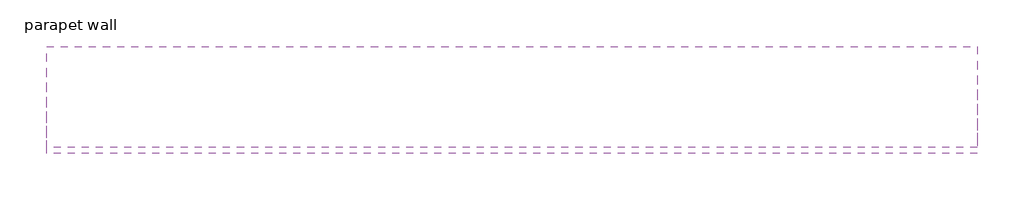
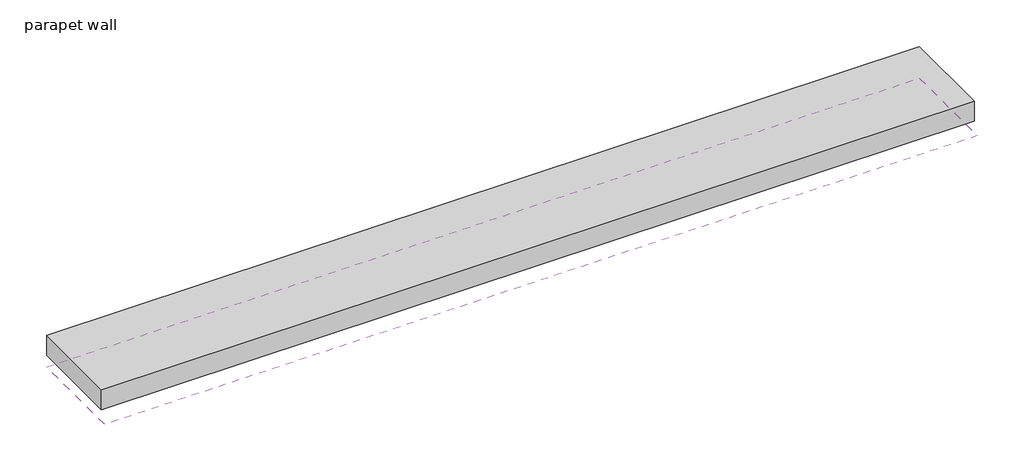
# One storey: 1 covering, 1 proxy.
"""IFC4 building model written with IfcOpenShell, lengths in millimetres."""

from ifc_helpers import new_model, si_unit, frame, origin, place, context, project, spatial, polyline, outline, extrude, transform, mapped, element, save
from components import generic_models_5_generic_models_5_1681292e

model = new_model("IFC4")

# Units and contexts
model_context = context("Model", 3, world=origin())
ifc_project = project(units=[si_unit("LENGTHUNIT", "METRE", prefix="MILLI")], contexts=[model_context])

# Site, building, storey
site = spatial("IfcSite", under=ifc_project)
building = spatial("IfcBuilding", under=site)
storey = spatial("IfcBuildingStorey", under=building, Name="parapet wall", Elevation=5029.2)

# Proxy
placement = place(None, origin())
generic_models_5_generic_models_5_shape = generic_models_5_generic_models_5_1681292e(model_context)
element("IfcBuildingElementProxy", 1, Name="Generic Models 5 : Generic Models 5", ObjectType="Generic Models 5 : Generic Models 5", at=placement, inside=storey, context=model_context, shape_type="MappedRepresentation", body=[
    mapped(generic_models_5_generic_models_5_shape, transform((0.0, 0.0, 0.0), x_axis=(1.0, 0.0, 0.0), y_axis=(0.0, 1.0, 0.0), z_axis=(0.0, 0.0, 1.0))),
])

# Covering
element("IfcCovering", 2, ObjectType="2' x 4' ACT System", at=placement, inside=storey, context=model_context, shape_type="SweptSolid", body=[
    extrude(outline(polyline([(-16168.5457338, -4852.8195077), (-20359.5457338, -4852.8195077), (-20359.5457338, -4370.2195077), (-16168.5457338, -4370.2195077), (-16168.5457338, -4852.8195077)])), frame((0.0, 0.0, 7467.6), z_axis=(0.0, 0.0, 1.0), x_axis=(1.0, 0.0, 0.0)), (0.0, 0.0, 1.0), 57.15),
])

save(model, "model.ifc")

# Revit data of these elements
# Type "2' x 4' ACT System"
#   Assembly Code = "C3030210"
#   built-in parameter 1002203 = 1 (stored number, unit not read)
#   built-in parameter 1002202 = 1 (stored number, unit not read)
#   Layers, outside or top first: 0' - 1 5/8" "Default" (function 1); 0' - 0 5/8" "Acoustic Ceiling Tile 24 x 48" (function 5)
# Element 1 (IfcBuildingElementProxy, "Generic Models 5 : Generic Models 5")
#   Phase Created = New Construction
# Element 2 (IfcCovering, "2' x 4' ACT System")
#   Height Offset From Level = 8' - 0"
#   Phase Created = New Construction
#   Materials on its faces: "Acoustic Ceiling Tile 24 x 48", "Default"
# Materials
#   "Default": colour RGB 127 127 127, transparency 0, Cost = 0
#   "Acoustic Ceiling Tile 24 x 48": class "Generic", colour RGB 229 229 229, transparency 0, Description = "Acoustic Ceiling Tile 24 x 48", Cost = 0
